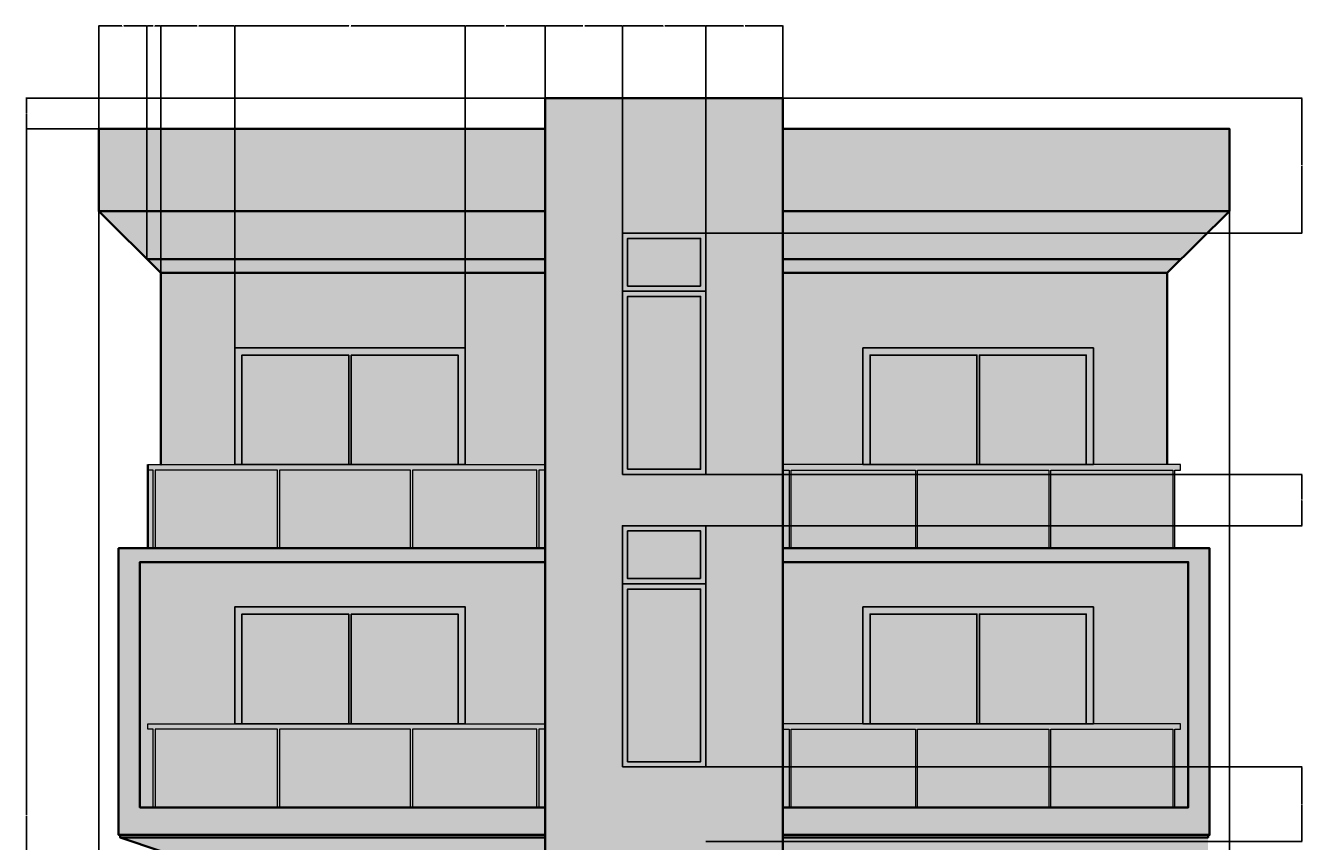
# Model space of a CAD drawing. Units: feet. Extents: x 2893 to 4112, y 897 to 1573.
# Tile 5 of 7: x 2893 to 3449, y 1217 to 1573. Entities that reach past the tile are written whole.
import ezdxf

# ---------------------------------------------------------------- set-up
doc = ezdxf.new("R2010")
doc.units = ezdxf.units.FT
for name, color, linetype, lineweight in [('A-ANNO-DIMS', 2, 'Continuous', 18), ('A-ELEV', 7, 'Continuous', 35), ('A-ELEV-PATT', 8, 'Continuous', 13), ('A-ELEV-RAIL', 4, 'Continuous', 18), ('A-GLAZ', 4, 'Continuous', 25)]:
    doc.layers.add(name, color=color, linetype=linetype, lineweight=lineweight)
doc.styles.get("Standard").update_dxf_attribs({"font": 'arial.ttf'})
doc.dimstyles.get("Standard").update_dxf_attribs({"dimtxt": 0.18, "dimasz": 0.18, "dimexe": 0.18, "dimexo": 0.0625, "dimgap": 0.09, "dimtad": 0, "dimtih": 1, "dimtoh": 1, "dimdec": 1, "dimzin": 0, "dimdsep": 46, "dimlunit": 3, "dimtxsty": 'Standard', "dimcen": 0.09, "dimadec": 0, "dimazin": 0, "dimtfac": 1, "dimtdec": 1, "dimtofl": 0, "dimtmove": 0, "dimatfit": 3, "dimfxl": 1, "dimtolj": 1, "dimtzin": 0, "dimarcsym": 0})

# ---------------------------------------------------------------- blocks, each defined once
blk = doc.blocks.new('WIN-SLIDING')
blk.add_lwpolyline([(100.48, 0), (0, 0), (0, 50.91), (100.48, 50.91)], close=True)
blk.add_lwpolyline([(100.48, 0), (0, 0), (0, 50.91), (100.48, 50.91)], close=True)
blk.add_lwpolyline([(97.33, 0), (97.33, 47.76), (50.81, 47.76), (50.81, 0), (49.67, 0), (49.67, 47.76), (3.15, 47.76), (3.15, 0)])
blk.add_lwpolyline([(97.33, 0), (97.33, 47.76), (50.81, 47.76), (50.81, 0), (49.67, 0), (49.67, 47.76), (3.15, 47.76), (3.15, 0)])
blk = doc.blocks.new('WIN-FEATURE')
for points in [[(36.35, 79.81), (0, 79.81), (0, 105.14), (36.35, 105.14)], [(36.35, 79.81), (0, 79.81), (0, 105.14), (36.35, 105.14)], [(34.08, 82.08), (2.27, 82.08), (2.27, 102.87), (34.08, 102.87)], [(34.08, 82.08), (2.27, 82.08), (2.27, 102.87), (34.08, 102.87)], [(0, 0), (36.35, 0), (36.35, 79.81), (0, 79.81)], [(0, 0), (36.35, 0), (36.35, 79.81), (0, 79.81)], [(2.27, 2.27), (34.08, 2.27), (34.08, 77.54), (2.27, 77.54)], [(2.27, 2.27), (34.08, 2.27), (34.08, 77.54), (2.27, 77.54)]]:
    blk.add_lwpolyline(points, close=True)
blk = doc.blocks.new('BALCONY-RAIL')
blk.add_lwpolyline([(56.56, 34.07), (3.3, 34.07), (3.3, 0), (2.43, 0), (2.43, 34.07), (0, 34.07), (0, 36.45), (173.25, 36.45), (173.25, 34.07), (170.48, 34.07), (170.48, 0), (169.61, 0), (169.61, 34.07), (115.47, 34.07), (115.47, 0), (114.59, 0), (114.59, 34.07), (57.43, 34.07), (57.43, 0), (56.56, 0)], close=True)
blk.add_lwpolyline([(56.56, 34.07), (3.3, 34.07), (3.3, 0), (2.43, 0), (2.43, 34.07), (0, 34.07), (0, 36.45), (173.25, 36.45), (173.25, 34.07), (170.48, 34.07), (170.48, 0), (169.61, 0), (169.61, 34.07), (115.47, 34.07), (115.47, 0), (114.59, 0), (114.59, 34.07), (57.43, 34.07), (57.43, 0), (56.56, 0)], close=True)
blk = doc.blocks.new('*D40')
at = {"layer": 'A-ANNO-DIMS', "color": 0, "lineweight": -2, "transparency": 16777216}
for p, q in [((2924.72, 1491.95), (2924.72, 1572.84)), ((2924.9, 1572.66), (2934.86, 1572.66)), ((2945.6, 1572.66), (2935.65, 1572.66)), ((2945.78, 1471.08), (2945.78, 1572.84))]:
    blk.add_line(p, q, dxfattribs=at)
at = {"layer": 'A-ANNO-DIMS', "color": 0, "transparency": 16777216}
for points in [[(2924.9, 1572.69), (2924.9, 1572.63), (2924.72, 1572.66)], [(2945.6, 1572.69), (2945.6, 1572.63), (2945.78, 1572.66)]]:
    blk.add_solid(points, dxfattribs=at)
at = {"layer": 'Defpoints', "color": 0, "transparency": 16777216}
for p in [(2945.78, 1572.66), (2924.72, 1491.89), (2945.78, 1471.01)]:
    blk.add_point(p, dxfattribs=at)
at = {"layer": 'A-ANNO-DIMS', "color": 0, "transparency": 16777216, "insert": (2935.25, 1572.66), "char_height": 0.18, "attachment_point": 5}
blk.add_mtext('\\A1;21.06', dxfattribs=at)
blk = doc.blocks.new('*D41')
at = {"layer": 'A-ANNO-DIMS', "color": 0, "lineweight": -2, "transparency": 16777216}
for p, q in [((2945.78, 1471.08), (2945.78, 1572.84)), ((2945.96, 1572.66), (2948.41, 1572.66)), ((2951.65, 1572.66), (2949.2, 1572.66)), ((2951.83, 1465.08), (2951.83, 1572.84))]:
    blk.add_line(p, q, dxfattribs=at)
at = {"layer": 'A-ANNO-DIMS', "color": 0, "transparency": 16777216}
for points in [[(2945.96, 1572.69), (2945.96, 1572.63), (2945.78, 1572.66)], [(2951.65, 1572.69), (2951.65, 1572.63), (2951.83, 1572.66)]]:
    blk.add_solid(points, dxfattribs=at)
at = {"layer": 'Defpoints', "color": 0, "transparency": 16777216}
for p in [(2951.83, 1572.66), (2945.78, 1471.01), (2951.83, 1465.01)]:
    blk.add_point(p, dxfattribs=at)
at = {"layer": 'A-ANNO-DIMS', "color": 0, "transparency": 16777216, "insert": (2948.81, 1572.66), "char_height": 0.18, "attachment_point": 5}
blk.add_mtext('\\A1;6.053', dxfattribs=at)
blk = doc.blocks.new('*D42')
at = {"layer": 'A-ANNO-DIMS', "color": 0, "lineweight": -2, "transparency": 16777216}
for p, q in [((2951.83, 1465.08), (2951.83, 1572.84)), ((2952.01, 1572.66), (2967.46, 1572.66)), ((2983.84, 1572.66), (2968.39, 1572.66)), ((2984.02, 1432.44), (2984.02, 1572.84))]:
    blk.add_line(p, q, dxfattribs=at)
at = {"layer": 'A-ANNO-DIMS', "color": 0, "transparency": 16777216}
for points in [[(2952.01, 1572.69), (2952.01, 1572.63), (2951.83, 1572.66)], [(2983.84, 1572.69), (2983.84, 1572.63), (2984.02, 1572.66)]]:
    blk.add_solid(points, dxfattribs=at)
at = {"layer": 'Defpoints', "color": 0, "transparency": 16777216}
for p in [(2984.02, 1572.66), (2951.83, 1465.01), (2984.02, 1432.38)]:
    blk.add_point(p, dxfattribs=at)
at = {"layer": 'A-ANNO-DIMS', "color": 0, "transparency": 16777216, "insert": (2967.93, 1572.66), "char_height": 0.18, "attachment_point": 5}
blk.add_mtext('\\A1;32.187', dxfattribs=at)
blk = doc.blocks.new('*D43')
at = {"layer": 'A-ANNO-DIMS', "color": 0, "lineweight": -2, "transparency": 16777216}
for p, q in [((2984.02, 1432.44), (2984.02, 1572.84)), ((2984.2, 1572.66), (3033.8, 1572.66)), ((3084.32, 1572.66), (3034.72, 1572.66)), ((3084.5, 1432.44), (3084.5, 1572.84))]:
    blk.add_line(p, q, dxfattribs=at)
at = {"layer": 'A-ANNO-DIMS', "color": 0, "transparency": 16777216}
for points in [[(2984.2, 1572.69), (2984.2, 1572.63), (2984.02, 1572.66)], [(3084.32, 1572.69), (3084.32, 1572.63), (3084.5, 1572.66)]]:
    blk.add_solid(points, dxfattribs=at)
at = {"layer": 'Defpoints', "color": 0, "transparency": 16777216}
for p in [(3084.5, 1572.66), (2984.02, 1432.38), (3084.5, 1432.38)]:
    blk.add_point(p, dxfattribs=at)
at = {"layer": 'A-ANNO-DIMS', "color": 0, "transparency": 16777216, "insert": (3034.26, 1572.66), "char_height": 0.18, "attachment_point": 5}
blk.add_mtext('\\A1;100.48', dxfattribs=at)
blk = doc.blocks.new('*D44')
at = {"layer": 'A-ANNO-DIMS', "color": 0, "lineweight": -2, "transparency": 16777216}
for p, q in [((3084.5, 1432.44), (3084.5, 1572.84)), ((3084.68, 1572.66), (3101.45, 1572.66)), ((3119.15, 1572.66), (3102.38, 1572.66)), ((3119.33, 1465.08), (3119.33, 1572.84))]:
    blk.add_line(p, q, dxfattribs=at)
at = {"layer": 'A-ANNO-DIMS', "color": 0, "transparency": 16777216}
for points in [[(3084.68, 1572.69), (3084.68, 1572.63), (3084.5, 1572.66)], [(3119.15, 1572.69), (3119.15, 1572.63), (3119.33, 1572.66)]]:
    blk.add_solid(points, dxfattribs=at)
at = {"layer": 'Defpoints', "color": 0, "transparency": 16777216}
for p in [(3119.33, 1572.66), (3119.33, 1465.01), (3084.5, 1432.38)]:
    blk.add_point(p, dxfattribs=at)
at = {"layer": 'A-ANNO-DIMS', "color": 0, "transparency": 16777216, "insert": (3101.91, 1572.66), "char_height": 0.18, "attachment_point": 5}
blk.add_mtext('\\A1;34.826', dxfattribs=at)
blk = doc.blocks.new('*D45')
at = {"layer": 'A-ANNO-DIMS', "color": 0, "lineweight": -2, "transparency": 16777216}
for p, q in [((3119.33, 1541.23), (3119.33, 1572.84)), ((3119.51, 1572.66), (3135.75, 1572.66)), ((3152.79, 1572.66), (3136.54, 1572.66)), ((3152.97, 1482.42), (3152.97, 1572.84))]:
    blk.add_line(p, q, dxfattribs=at)
at = {"layer": 'A-ANNO-DIMS', "color": 0, "transparency": 16777216}
for points in [[(3119.51, 1572.69), (3119.51, 1572.63), (3119.33, 1572.66)], [(3152.79, 1572.69), (3152.79, 1572.63), (3152.97, 1572.66)]]:
    blk.add_solid(points, dxfattribs=at)
at = {"layer": 'Defpoints', "color": 0, "transparency": 16777216}
for p in [(3152.97, 1572.66), (3119.33, 1541.16), (3152.97, 1482.36)]:
    blk.add_point(p, dxfattribs=at)
at = {"layer": 'A-ANNO-DIMS', "color": 0, "transparency": 16777216, "insert": (3136.15, 1572.66), "char_height": 0.18, "attachment_point": 5}
blk.add_mtext('\\A1;33.64', dxfattribs=at)
blk = doc.blocks.new('*D46')
at = {"layer": 'A-ANNO-DIMS', "color": 0, "lineweight": -2, "transparency": 16777216}
for p, q in [((3152.97, 1482.42), (3152.97, 1572.84)), ((3153.15, 1572.66), (3170.75, 1572.66)), ((3189.14, 1572.66), (3171.54, 1572.66)), ((3189.32, 1482.42), (3189.32, 1572.84))]:
    blk.add_line(p, q, dxfattribs=at)
at = {"layer": 'A-ANNO-DIMS', "color": 0, "transparency": 16777216}
for points in [[(3153.15, 1572.69), (3153.15, 1572.63), (3152.97, 1572.66)], [(3189.14, 1572.69), (3189.14, 1572.63), (3189.32, 1572.66)]]:
    blk.add_solid(points, dxfattribs=at)
at = {"layer": 'Defpoints', "color": 0, "transparency": 16777216}
for p in [(3189.32, 1572.66), (3152.97, 1482.36), (3189.32, 1482.36)]:
    blk.add_point(p, dxfattribs=at)
at = {"layer": 'A-ANNO-DIMS', "color": 0, "transparency": 16777216, "insert": (3171.14, 1572.66), "char_height": 0.18, "attachment_point": 5}
blk.add_mtext('\\A1;36.35', dxfattribs=at)
blk = doc.blocks.new('*D47')
at = {"layer": 'A-ANNO-DIMS', "color": 0, "lineweight": -2, "transparency": 16777216}
for p, q in [((3189.32, 1482.42), (3189.32, 1572.84)), ((3189.5, 1572.66), (3205.74, 1572.66)), ((3222.78, 1572.66), (3206.53, 1572.66)), ((3222.96, 1541.23), (3222.96, 1572.84))]:
    blk.add_line(p, q, dxfattribs=at)
at = {"layer": 'A-ANNO-DIMS', "color": 0, "transparency": 16777216}
for points in [[(3189.5, 1572.69), (3189.5, 1572.63), (3189.32, 1572.66)], [(3222.78, 1572.69), (3222.78, 1572.63), (3222.96, 1572.66)]]:
    blk.add_solid(points, dxfattribs=at)
at = {"layer": 'Defpoints', "color": 0, "transparency": 16777216}
for p in [(3222.96, 1572.66), (3222.96, 1541.16), (3189.32, 1482.36)]:
    blk.add_point(p, dxfattribs=at)
at = {"layer": 'A-ANNO-DIMS', "color": 0, "transparency": 16777216, "insert": (3206.14, 1572.66), "char_height": 0.18, "attachment_point": 5}
blk.add_mtext('\\A1;33.64', dxfattribs=at)
blk = doc.blocks.new('*D48')
at = {"layer": 'A-ANNO-DIMS', "color": 0, "lineweight": -2, "transparency": 16777216}
for p, q in [((2924.72, 1491.83), (2924.72, 897.37)), ((3417.56, 1491.83), (3417.56, 897.37)), ((2924.9, 897.55), (3170.74, 897.55)), ((3417.38, 897.55), (3171.54, 897.55))]:
    blk.add_line(p, q, dxfattribs=at)
at = {"layer": 'A-ANNO-DIMS', "color": 0, "transparency": 16777216}
for points in [[(2924.9, 897.58), (2924.9, 897.52), (2924.72, 897.55)], [(3417.38, 897.58), (3417.38, 897.52), (3417.56, 897.55)]]:
    blk.add_solid(points, dxfattribs=at)
at = {"layer": 'Defpoints', "color": 0, "transparency": 16777216}
for p in [(2924.72, 1491.89), (3417.56, 1491.89), (3417.56, 897.55)]:
    blk.add_point(p, dxfattribs=at)
at = {"layer": 'A-ANNO-DIMS', "color": 0, "transparency": 16777216, "insert": (3171.14, 897.55), "char_height": 0.18, "attachment_point": 5}
blk.add_mtext('\\A1;492.8', dxfattribs=at)
blk = doc.blocks.new('*D52')
at = {"layer": 'A-ANNO-DIMS', "color": 0, "lineweight": -2, "transparency": 16777216}
for p, q in [((3189.38, 1249.71), (3449.24, 1249.71)), ((3449.06, 1249.53), (3449.06, 1233.66)), ((3449.06, 1217.43), (3449.06, 1233.29)), ((3189.38, 1217.25), (3449.24, 1217.25))]:
    blk.add_line(p, q, dxfattribs=at)
at = {"layer": 'A-ANNO-DIMS', "color": 0, "transparency": 16777216}
for points in [[(3449.03, 1249.53), (3449.09, 1249.53), (3449.06, 1249.71)], [(3449.03, 1217.43), (3449.09, 1217.43), (3449.06, 1217.25)]]:
    blk.add_solid(points, dxfattribs=at)
at = {"layer": 'Defpoints', "color": 0, "transparency": 16777216}
for p in [(3189.32, 1249.71), (3449.06, 1249.71), (3189.32, 1217.25)]:
    blk.add_point(p, dxfattribs=at)
at = {"layer": 'A-ANNO-DIMS', "color": 0, "transparency": 16777216, "insert": (3449.06, 1233.48), "char_height": 0.18, "attachment_point": 5}
blk.add_mtext('\\A1;32.46', dxfattribs=at)
blk = doc.blocks.new('*D53')
at = {"layer": 'A-ANNO-DIMS', "color": 0, "lineweight": -2, "transparency": 16777216}
for p, q in [((3189.38, 1377.22), (3449.24, 1377.22)), ((3449.06, 1377.04), (3449.06, 1366.22)), ((3449.06, 1355.02), (3449.06, 1365.85)), ((3189.38, 1354.84), (3449.24, 1354.84))]:
    blk.add_line(p, q, dxfattribs=at)
at = {"layer": 'A-ANNO-DIMS', "color": 0, "transparency": 16777216}
for points in [[(3449.03, 1377.04), (3449.09, 1377.04), (3449.06, 1377.22)], [(3449.03, 1355.02), (3449.09, 1355.02), (3449.06, 1354.84)]]:
    blk.add_solid(points, dxfattribs=at)
at = {"layer": 'Defpoints', "color": 0, "transparency": 16777216}
for p in [(3189.32, 1377.22), (3449.06, 1377.22), (3189.32, 1354.84)]:
    blk.add_point(p, dxfattribs=at)
at = {"layer": 'A-ANNO-DIMS', "color": 0, "transparency": 16777216, "insert": (3449.06, 1366.03), "char_height": 0.18, "attachment_point": 5}
blk.add_mtext('\\A1;22.38', dxfattribs=at)
blk = doc.blocks.new('*D54')
at = {"layer": 'A-ANNO-DIMS', "color": 0, "lineweight": -2, "transparency": 16777216}
for p, q in [((3223.02, 1541.16), (3449.24, 1541.16)), ((3449.06, 1540.98), (3449.06, 1511.95)), ((3449.06, 1482.54), (3449.06, 1511.58)), ((3189.38, 1482.36), (3449.24, 1482.36))]:
    blk.add_line(p, q, dxfattribs=at)
at = {"layer": 'A-ANNO-DIMS', "color": 0, "transparency": 16777216}
for points in [[(3449.03, 1540.98), (3449.09, 1540.98), (3449.06, 1541.16)], [(3449.03, 1482.54), (3449.09, 1482.54), (3449.06, 1482.36)]]:
    blk.add_solid(points, dxfattribs=at)
at = {"layer": 'Defpoints', "color": 0, "transparency": 16777216}
for p in [(3222.96, 1541.16), (3449.06, 1541.16), (3189.32, 1482.36)]:
    blk.add_point(p, dxfattribs=at)
at = {"layer": 'A-ANNO-DIMS', "color": 0, "transparency": 16777216, "insert": (3449.06, 1511.76), "char_height": 0.18, "attachment_point": 5}
blk.add_mtext('\\A1;58.8', dxfattribs=at)
blk = doc.blocks.new('*D55')
at = {"layer": 'A-ANNO-DIMS', "color": 0, "lineweight": -2, "transparency": 16777216}
for p, q in [((2924.66, 1527.89), (2893.04, 1527.89)), ((2893.22, 1527.71), (2893.22, 1228.65)), ((2893.22, 929.23), (2893.22, 1228.29)), ((2926.44, 929.05), (2893.04, 929.05))]:
    blk.add_line(p, q, dxfattribs=at)
at = {"layer": 'A-ANNO-DIMS', "color": 0, "transparency": 16777216}
for points in [[(2893.19, 1527.71), (2893.25, 1527.71), (2893.22, 1527.89)], [(2893.19, 929.23), (2893.25, 929.23), (2893.22, 929.05)]]:
    blk.add_solid(points, dxfattribs=at)
at = {"layer": 'Defpoints', "color": 0, "transparency": 16777216}
for p in [(2893.22, 1527.89), (2924.72, 1527.89), (2926.51, 929.05)]:
    blk.add_point(p, dxfattribs=at)
at = {"layer": 'A-ANNO-DIMS', "color": 0, "transparency": 16777216, "insert": (2893.22, 1228.47), "char_height": 0.18, "attachment_point": 5}
blk.add_mtext('\\A1;598.8', dxfattribs=at)
blk = doc.blocks.new('*D56')
at = {"layer": 'A-ANNO-DIMS', "color": 0, "lineweight": -2, "transparency": 16777216}
for p, q in [((3119.26, 1541.16), (2893.04, 1541.16)), ((2893.22, 1540.98), (2893.22, 1534.71)), ((2893.22, 1528.07), (2893.22, 1534.34)), ((2924.66, 1527.89), (2893.04, 1527.89))]:
    blk.add_line(p, q, dxfattribs=at)
at = {"layer": 'A-ANNO-DIMS', "color": 0, "transparency": 16777216}
for points in [[(2893.19, 1540.98), (2893.25, 1540.98), (2893.22, 1541.16)], [(2893.19, 1528.07), (2893.25, 1528.07), (2893.22, 1527.89)]]:
    blk.add_solid(points, dxfattribs=at)
at = {"layer": 'Defpoints', "color": 0, "transparency": 16777216}
for p in [(3119.33, 1541.16), (2893.22, 1527.89), (2924.72, 1527.89)]:
    blk.add_point(p, dxfattribs=at)
at = {"layer": 'A-ANNO-DIMS', "color": 0, "transparency": 16777216, "insert": (2893.22, 1534.53), "char_height": 0.18, "attachment_point": 5}
blk.add_mtext('\\A1;13.276', dxfattribs=at)

msp = doc.modelspace()

# ---------------------------------------------------------------- hatches: boundary and pattern name
at = {"layer": 'A-ELEV-PATT'}
h = msp.add_hatch(color=256, dxfattribs=at)
h.dxf.hatch_style = 1
h.paths.add_polyline_path([(3222.9589, 1541.1646), (3119.3255, 1541.1646), (3119.3255, 967.0143), (3127.3151, 967.0143), (3127.3151, 1087.0143), (3214.9693, 1087.0143), (3214.9693, 1078.6766), (3214.9693, 967.0143), (3222.9589, 967.0143)])
h.paths.add_polyline_path([(3152.9675, 1482.3616), (3189.3169, 1482.3616), (3189.3169, 1457.0324), (3189.3169, 1377.2236), (3152.9675, 1377.2236), (3152.9675, 1457.0324)], flags=16)
h.paths.add_polyline_path([(3155.237, 1480.0922), (3187.0474, 1480.0922), (3187.0474, 1459.3019), (3155.237, 1459.3019)], flags=0)
h.paths.add_polyline_path([(3155.237, 1454.7629), (3187.0474, 1454.7629), (3187.0474, 1379.4931), (3155.237, 1379.4931)], flags=0)
h.paths.add_polyline_path([(3152.9675, 1354.8437), (3189.3169, 1354.8437), (3189.3169, 1329.5145), (3189.3169, 1249.7057), (3152.9675, 1249.7057), (3152.9675, 1329.5145)], flags=16)
h.paths.add_polyline_path([(3155.237, 1352.5742), (3187.0474, 1352.5742), (3187.0474, 1331.784), (3155.237, 1331.784)], flags=0)
h.paths.add_polyline_path([(3155.237, 1327.245), (3187.0474, 1327.245), (3187.0474, 1251.9752), (3155.237, 1251.9752)], flags=0)
h.paths.add_polyline_path([(3152.9675, 1217.2478), (3189.3169, 1217.2478), (3189.3169, 1191.9186), (3189.3169, 1112.1098), (3152.9675, 1112.1098), (3152.9675, 1191.9186)], flags=16)
h.paths.add_polyline_path([(3155.237, 1214.9783), (3187.0474, 1214.9783), (3187.0474, 1194.1881), (3155.237, 1194.1881)], flags=0)
h.paths.add_polyline_path([(3155.237, 1189.6491), (3187.0474, 1189.6491), (3187.0474, 1114.3793), (3155.237, 1114.3793)], flags=0)
h = msp.add_hatch(dxfattribs=at)
h.set_pattern_fill('AR-BRELM', color=256, scale=0.1)
h.set_pattern_definition([(0, (-663.002, 0), (0, 13.5484), [19.3675, -0.9525]), (0, (-663.002, 5.715), (0, 13.5484), [19.3675, -0.9525]), (0, (-657.922, 6.774), (0, 13.5484), [9.2075, -0.9525]), (0, (-657.922, 12.489), (0, 13.5484), [9.2075, -0.9525]), (90, (-663.002, 0), (-20.32, 1e-15), [5.715, -7.8334]), (90, (-663.954, 0), (-20.32, 1e-15), [5.715, -7.8334]), (90, (-657.922, 6.774), (-10.16, 6e-16), [5.715, -7.8334]), (90, (-658.874, 6.774), (-10.16, 6e-16), [5.715, -7.8334])])
h.paths.add_polyline_path([(3222.9589, 1541.1646), (3119.3255, 1541.1646), (3119.3255, 967.0143), (3127.3151, 967.0143), (3127.3151, 1087.0143), (3214.9693, 1087.0143), (3214.9693, 1078.6766), (3214.9693, 967.0143), (3222.9589, 967.0143)])
h.paths.add_polyline_path([(3152.9675, 1482.3616), (3189.3169, 1482.3616), (3189.3169, 1457.0324), (3189.3169, 1377.2236), (3152.9675, 1377.2236), (3152.9675, 1457.0324)], flags=16)
h.paths.add_polyline_path([(3155.237, 1480.0922), (3187.0474, 1480.0922), (3187.0474, 1459.3019), (3155.237, 1459.3019)], flags=0)
h.paths.add_polyline_path([(3155.237, 1454.7629), (3187.0474, 1454.7629), (3187.0474, 1379.4931), (3155.237, 1379.4931)], flags=0)
h.paths.add_polyline_path([(3152.9675, 1354.8437), (3189.3169, 1354.8437), (3189.3169, 1329.5145), (3189.3169, 1249.7057), (3152.9675, 1249.7057), (3152.9675, 1329.5145)], flags=16)
h.paths.add_polyline_path([(3155.237, 1352.5742), (3187.0474, 1352.5742), (3187.0474, 1331.784), (3155.237, 1331.784)], flags=0)
h.paths.add_polyline_path([(3155.237, 1327.245), (3187.0474, 1327.245), (3187.0474, 1251.9752), (3155.237, 1251.9752)], flags=0)
h.paths.add_polyline_path([(3152.9675, 1217.2478), (3189.3169, 1217.2478), (3189.3169, 1191.9186), (3189.3169, 1112.1098), (3152.9675, 1112.1098), (3152.9675, 1191.9186)], flags=16)
h.paths.add_polyline_path([(3155.237, 1214.9783), (3187.0474, 1214.9783), (3187.0474, 1194.1881), (3155.237, 1194.1881)], flags=0)
h.paths.add_polyline_path([(3155.237, 1189.6491), (3187.0474, 1189.6491), (3187.0474, 1114.3793), (3155.237, 1114.3793)], flags=0)
h = msp.add_hatch(color=256, dxfattribs=at)
h.dxf.hatch_style = 1
h.paths.add_polyline_path([(3119.3255, 1527.889), (2924.7207, 1527.889), (2924.7207, 1491.889), (3119.3255, 1491.889)])
h.paths.add_polyline_path([(3417.5637, 1527.889), (3222.9589, 1527.889), (3222.9589, 1491.889), (3417.5637, 1491.889)])
h.paths.add_polyline_path([(3119.3255, 1102.9302), (2946.0771, 1102.9302), (2946.0771, 1139.3799), (2934.0287, 1139.3799), (2934.0287, 1093.0143), (3119.3255, 1093.0143)])
h.paths.add_polyline_path([(3119.3255, 1093.0143), (2934.4679, 1093.0143), (2934.4679, 1087.0143), (3119.3255, 1087.0143)])
h.paths.add_polyline_path([(3408.2557, 1139.3799), (3396.2073, 1139.3799), (3396.2073, 1136.9984), (3396.2073, 1102.9302), (3222.9589, 1102.9302), (3222.9589, 1093.0143), (3408.2557, 1093.0143)])
h.paths.add_polyline_path([(3407.8165, 1093.0143), (3222.9589, 1093.0143), (3222.9589, 1087.0143), (3407.8165, 1087.0143)])
h = msp.add_hatch(color=256, dxfattribs=at)
h.dxf.hatch_style = 1
h.paths.add_polyline_path([(3119.3255, 1491.889), (2924.7207, 1491.889), (2945.7801, 1471.0143), (3119.3255, 1471.0143)])
h.paths.add_polyline_path([(3119.3255, 1471.0143), (2945.7801, 1471.0143), (2951.8333, 1465.0143), (3119.3255, 1465.0143)])
h.paths.add_polyline_path([(3119.3255, 1465.0143), (2951.8333, 1465.0143), (2951.8333, 1381.4641), (2984.02, 1381.4641), (2984.02, 1432.3761), (3084.4999, 1432.3761), (3084.4999, 1381.4641), (3119.3255, 1381.4641)])
h.paths.add_polyline_path([(3417.5637, 1491.889), (3222.9589, 1491.889), (3222.9589, 1471.0143), (3396.5042, 1471.0143)])
h.paths.add_polyline_path([(3396.5042, 1471.0143), (3222.9589, 1471.0143), (3222.9589, 1465.0143), (3390.4511, 1465.0143)])
h.paths.add_polyline_path([(3390.4511, 1465.0143), (3222.9589, 1465.0143), (3222.9589, 1381.4641), (3257.7845, 1381.4641), (3257.7845, 1432.3761), (3358.2644, 1432.3761), (3358.2644, 1381.4641), (3390.4511, 1381.4641)])
h.paths.add_polyline_path([(3119.3255, 1339.0143), (2942.6825, 1339.0143), (2942.6825, 1232.1197), (2948.5078, 1232.1197), (2948.5078, 1266.188), (2946.0771, 1266.188), (2946.0771, 1268.5695), (2984.02, 1268.5695), (2984.02, 1319.4815), (3084.4999, 1319.4815), (3084.4999, 1268.5695), (3119.3255, 1268.5695)], flags=17)
h.paths.add_polyline_path([(3399.6019, 1339.0143), (3222.9589, 1339.0143), (3222.9589, 1268.5695), (3257.7845, 1268.5695), (3257.7845, 1319.4815), (3358.2644, 1319.4815), (3358.2644, 1268.5695), (3396.2073, 1268.5695), (3396.2073, 1266.188), (3393.7766, 1266.188), (3393.7766, 1232.1197), (3399.6019, 1232.1197)], flags=17)
h.paths.add_polyline_path([(2942.6825, 1339.0143), (3119.3255, 1339.0143), (3119.3255, 1345.0143), (2933.3946, 1345.0143), (2933.3946, 1232.1197), (2933.3946, 1220.0947), (3119.3255, 1220.0947), (3119.3255, 1232.1197), (2942.6825, 1232.1197)])
h.paths.add_polyline_path([(3408.8898, 1345.0143), (3222.9589, 1345.0143), (3222.9589, 1339.0143), (3399.6019, 1339.0143), (3399.6019, 1232.1197), (3393.7766, 1232.1197), (3392.9028, 1232.1197), (3222.9589, 1232.1197), (3222.9589, 1220.0947), (3408.8898, 1220.0947), (3408.8898, 1232.1197)])
h.paths.add_polyline_path([(2984.02, 1190.2919), (3084.4999, 1190.2919), (3084.4999, 1139.3799), (3119.3255, 1139.3799), (3119.3255, 1213.0143), (2951.8333, 1213.0143), (2951.8333, 1139.3799), (2984.02, 1139.3799)])
h.paths.add_polyline_path([(3119.3255, 1219.0143), (2934.0287, 1219.0143), (2951.8333, 1213.0143), (3119.3255, 1213.0143)])
h.paths.add_polyline_path([(3390.4511, 1213.0143), (3222.9589, 1213.0143), (3222.9589, 1139.3799), (3257.7845, 1139.3799), (3257.7845, 1190.2919), (3358.2644, 1190.2919), (3358.2644, 1139.3799), (3390.4511, 1139.3799)])
h.paths.add_polyline_path([(3408.2557, 1219.0143), (3222.9589, 1219.0143), (3222.9589, 1213.0143), (3408.2557, 1213.0143)])
h = msp.add_hatch(color=256, dxfattribs=at)
h.dxf.hatch_style = 1
h.paths.add_polyline_path([(3119.3255, 1139.3799), (2946.0771, 1139.3799), (2946.0771, 1136.9984), (2948.5078, 1136.9984), (2948.5078, 1102.9302), (2949.3816, 1102.9302), (2949.3816, 1136.9984), (3002.6337, 1136.9984), (3002.6337, 1102.9302), (3003.5075, 1102.9302), (3003.5075, 1136.9984), (3060.6708, 1136.9984), (3060.6708, 1102.9302), (3061.5445, 1102.9302), (3061.5445, 1136.9984), (3115.685, 1136.9984), (3115.685, 1102.9302), (3116.5588, 1102.9302), (3116.5588, 1136.9984), (3119.3255, 1136.9984)])
h.paths.add_polyline_path([(2987.1701, 1187.1419), (3033.6877, 1187.1419), (3033.6877, 1139.3799), (3034.8322, 1139.3799), (3034.8322, 1187.1419), (3081.3499, 1187.1419), (3081.3499, 1139.3799), (3084.4999, 1139.3799), (3084.4999, 1190.2919), (2984.02, 1190.2919), (2984.02, 1139.3799), (2987.1701, 1139.3799)])
h.paths.add_polyline_path([(2987.1701, 1316.3314), (3033.6877, 1316.3314), (3033.6877, 1268.5695), (3034.8322, 1268.5695), (3034.8322, 1316.3314), (3081.3499, 1316.3314), (3081.3499, 1268.5695), (3084.4999, 1268.5695), (3084.4999, 1319.4815), (2984.02, 1319.4815), (2984.02, 1268.5695), (2987.1701, 1268.5695)])
h.paths.add_polyline_path([(3003.5075, 1266.188), (3060.6708, 1266.188), (3060.6708, 1232.1197), (3061.5445, 1232.1197), (3061.5445, 1266.188), (3115.685, 1266.188), (3115.685, 1232.1197), (3116.5588, 1232.1197), (3116.5588, 1266.188), (3119.3255, 1266.188), (3119.3255, 1268.5695), (2946.0771, 1268.5695), (2946.0771, 1266.188), (2948.5078, 1266.188), (2948.5078, 1232.1197), (2949.3816, 1232.1197), (2949.3816, 1266.188), (3002.6337, 1266.188), (3002.6337, 1232.1197), (3003.5075, 1232.1197)])
h.paths.add_polyline_path([(2987.1701, 1429.226), (3033.6877, 1429.226), (3033.6877, 1381.4641), (3034.8322, 1381.4641), (3034.8322, 1429.226), (3081.3499, 1429.226), (3081.3499, 1381.4641), (3084.4999, 1381.4641), (3084.4999, 1432.3761), (2984.02, 1432.3761), (2984.02, 1381.4641), (2987.1701, 1381.4641)])
h.paths.add_polyline_path([(3119.3255, 1381.4641), (2946.0771, 1381.4641), (2946.0771, 1379.0826), (2948.5078, 1379.0826), (2948.5078, 1345.0143), (2949.3816, 1345.0143), (2949.3816, 1379.0826), (3002.6337, 1379.0826), (3002.6337, 1345.0143), (3003.5075, 1345.0143), (3003.5075, 1379.0826), (3060.6708, 1379.0826), (3060.6708, 1345.0143), (3061.5445, 1345.0143), (3061.5445, 1379.0826), (3115.685, 1379.0826), (3115.685, 1345.0143), (3116.5588, 1345.0143), (3116.5588, 1379.0826), (3119.3255, 1379.0826)])
h.paths.add_polyline_path([(3189.3169, 1482.3616), (3152.9675, 1482.3616), (3152.9675, 1457.0324), (3189.3169, 1457.0324)])
h.paths.add_polyline_path([(3155.237, 1480.0922), (3187.0474, 1480.0922), (3187.0474, 1459.3019), (3155.237, 1459.3019)], flags=16)
h.paths.add_polyline_path([(3189.3169, 1457.0324), (3152.9675, 1457.0324), (3152.9675, 1377.2236), (3189.3169, 1377.2236)])
h.paths.add_polyline_path([(3155.237, 1454.7629), (3187.0474, 1454.7629), (3187.0474, 1379.4931), (3155.237, 1379.4931)], flags=16)
h.paths.add_polyline_path([(3358.2644, 1432.3761), (3257.7845, 1432.3761), (3257.7845, 1381.4641), (3260.9345, 1381.4641), (3260.9345, 1429.226), (3307.4522, 1429.226), (3307.4522, 1381.4641), (3308.5967, 1381.4641), (3308.5967, 1429.226), (3355.1143, 1429.226), (3355.1143, 1381.4641), (3358.2644, 1381.4641)])
h.paths.add_polyline_path([(3396.2073, 1381.4641), (3222.9589, 1381.4641), (3222.9589, 1379.0826), (3225.7256, 1379.0826), (3225.7256, 1345.0143), (3226.5994, 1345.0143), (3226.5994, 1379.0826), (3280.7398, 1379.0826), (3280.7398, 1345.0143), (3281.6136, 1345.0143), (3281.6136, 1379.0826), (3338.7769, 1379.0826), (3338.7769, 1345.0143), (3339.6507, 1345.0143), (3339.6507, 1379.0826), (3392.9028, 1379.0826), (3392.9028, 1345.0143), (3393.7766, 1345.0143), (3393.7766, 1379.0826), (3396.2073, 1379.0826)])
h.paths.add_polyline_path([(3358.2644, 1319.4815), (3257.7845, 1319.4815), (3257.7845, 1268.5695), (3260.9345, 1268.5695), (3260.9345, 1316.3314), (3307.4522, 1316.3314), (3307.4522, 1268.5695), (3308.5967, 1268.5695), (3308.5967, 1316.3314), (3355.1143, 1316.3314), (3355.1143, 1268.5695), (3358.2644, 1268.5695)])
h.paths.add_polyline_path([(3396.2073, 1268.5695), (3222.9589, 1268.5695), (3222.9589, 1266.188), (3225.7256, 1266.188), (3225.7256, 1232.1197), (3226.5994, 1232.1197), (3226.5994, 1266.188), (3280.7398, 1266.188), (3280.7398, 1232.1197), (3281.6136, 1232.1197), (3281.6136, 1266.188), (3338.7769, 1266.188), (3338.7769, 1232.1197), (3339.6507, 1232.1197), (3339.6507, 1266.188), (3392.9028, 1266.188), (3392.9028, 1232.1197), (3393.7766, 1232.1197), (3393.7766, 1266.188), (3396.2073, 1266.188)])
h.paths.add_polyline_path([(3260.9345, 1187.1419), (3307.4522, 1187.1419), (3307.4522, 1139.3799), (3308.5967, 1139.3799), (3308.5967, 1187.1419), (3355.1143, 1187.1419), (3355.1143, 1139.3799), (3358.2644, 1139.3799), (3358.2644, 1190.2919), (3257.7845, 1190.2919), (3257.7845, 1139.3799), (3260.9345, 1139.3799)])
h.paths.add_polyline_path([(3396.2073, 1139.3799), (3222.9589, 1139.3799), (3222.9589, 1136.9984), (3225.7256, 1136.9984), (3225.7256, 1102.9302), (3226.5994, 1102.9302), (3226.5994, 1136.9984), (3280.7398, 1136.9984), (3280.7398, 1102.9302), (3281.6136, 1102.9302), (3281.6136, 1136.9984), (3338.7769, 1136.9984), (3338.7769, 1102.9302), (3339.6507, 1102.9302), (3339.6507, 1136.9984), (3392.9028, 1136.9984), (3392.9028, 1102.9302), (3393.7766, 1102.9302), (3393.7766, 1136.9984), (3396.2073, 1136.9984)])
h.paths.add_polyline_path([(3189.3169, 1354.8437), (3152.9675, 1354.8437), (3152.9675, 1329.5145), (3189.3169, 1329.5145)])
h.paths.add_polyline_path([(3155.237, 1331.784), (3155.237, 1352.5742), (3187.0474, 1352.5742), (3187.0474, 1331.784)], flags=16)
h.paths.add_polyline_path([(3189.3169, 1329.5145), (3152.9675, 1329.5145), (3152.9675, 1249.7057), (3189.3169, 1249.7057)])
h.paths.add_polyline_path([(3155.237, 1327.245), (3187.0474, 1327.245), (3187.0474, 1251.9752), (3155.237, 1251.9752)], flags=16)
h.paths.add_polyline_path([(3189.3169, 1191.9186), (3152.9675, 1191.9186), (3152.9675, 1112.1098), (3189.3169, 1112.1098)])
h.paths.add_polyline_path([(3155.237, 1189.6491), (3187.0474, 1189.6491), (3187.0474, 1114.3793), (3155.237, 1114.3793)], flags=16)
h.paths.add_polyline_path([(3189.3169, 1217.2478), (3152.9675, 1217.2478), (3152.9675, 1191.9186), (3189.3169, 1191.9186)])
h.paths.add_polyline_path([(3155.237, 1194.1881), (3155.237, 1214.9783), (3187.0474, 1214.9783), (3187.0474, 1194.1881)], flags=16)
h = msp.add_hatch(color=256, dxfattribs=at)
h.dxf.hatch_style = 1
h.paths.add_polyline_path([(3033.6877, 1429.226), (2987.1701, 1429.226), (2987.1701, 1381.4641), (3033.6877, 1381.4641)])
h.paths.add_polyline_path([(3081.3499, 1429.226), (3034.8322, 1429.226), (3034.8322, 1381.4641), (3081.3499, 1381.4641)])
h.paths.add_polyline_path([(3115.685, 1379.0826), (3061.5445, 1379.0826), (3061.5445, 1345.0143), (3115.685, 1345.0143)])
h.paths.add_polyline_path([(3119.3255, 1379.0826), (3116.5588, 1379.0826), (3116.5588, 1345.0143), (3119.3255, 1345.0143)])
h.paths.add_polyline_path([(3060.6708, 1379.0826), (3003.5075, 1379.0826), (3003.5075, 1345.0143), (3060.6708, 1345.0143)])
h.paths.add_polyline_path([(3002.6337, 1379.0826), (2949.3816, 1379.0826), (2949.3816, 1345.0143), (3002.6337, 1345.0143)])
h.paths.add_polyline_path([(2948.5078, 1379.0826), (2946.0771, 1379.0826), (2946.0771, 1345.0143), (2948.5078, 1345.0143)])
h.paths.add_polyline_path([(3355.1143, 1429.226), (3308.5967, 1429.226), (3308.5967, 1381.4641), (3355.1143, 1381.4641)])
h.paths.add_polyline_path([(3307.4522, 1429.226), (3260.9345, 1429.226), (3260.9345, 1381.4641), (3307.4522, 1381.4641)])
h.paths.add_polyline_path([(3225.7256, 1379.0826), (3222.9589, 1379.0826), (3222.9589, 1345.0143), (3225.7256, 1345.0143)])
h.paths.add_polyline_path([(3280.7398, 1379.0826), (3226.5994, 1379.0826), (3226.5994, 1345.0143), (3280.7398, 1345.0143)])
h.paths.add_polyline_path([(3338.7769, 1379.0826), (3281.6136, 1379.0826), (3281.6136, 1345.0143), (3338.7769, 1345.0143)])
h.paths.add_polyline_path([(3392.9028, 1379.0826), (3339.6507, 1379.0826), (3339.6507, 1345.0143), (3392.9028, 1345.0143)])
h.paths.add_polyline_path([(3187.0474, 1480.0922), (3155.237, 1480.0922), (3155.237, 1459.3019), (3187.0474, 1459.3019)])
h.paths.add_polyline_path([(3187.0474, 1454.7629), (3155.237, 1454.7629), (3155.237, 1379.4931), (3187.0474, 1379.4931)])
h.paths.add_polyline_path([(3187.0474, 1352.5742), (3155.237, 1352.5742), (3155.237, 1331.784), (3187.0474, 1331.784)])
h.paths.add_polyline_path([(3187.0474, 1327.245), (3155.237, 1327.245), (3155.237, 1251.9752), (3187.0474, 1251.9752)])
h.paths.add_polyline_path([(3033.6877, 1316.3314), (2987.1701, 1316.3314), (2987.1701, 1268.5695), (3033.6877, 1268.5695)])
h.paths.add_polyline_path([(3081.3499, 1316.3314), (3034.8322, 1316.3314), (3034.8322, 1268.5695), (3081.3499, 1268.5695)])
h.paths.add_polyline_path([(3002.6337, 1266.188), (2949.3816, 1266.188), (2949.3816, 1232.1197), (3002.6337, 1232.1197)])
h.paths.add_polyline_path([(3060.6708, 1266.188), (3003.5075, 1266.188), (3003.5075, 1232.1197), (3060.6708, 1232.1197)])
h.paths.add_polyline_path([(3115.685, 1266.188), (3061.5445, 1266.188), (3061.5445, 1232.1197), (3115.685, 1232.1197)])
h.paths.add_polyline_path([(3119.3255, 1266.188), (3116.5588, 1266.188), (3116.5588, 1232.1197), (3119.3255, 1232.1197)])
h.paths.add_polyline_path([(3307.4522, 1316.3314), (3260.9345, 1316.3314), (3260.9345, 1268.5695), (3307.4522, 1268.5695)])
h.paths.add_polyline_path([(3355.1143, 1316.3314), (3308.5967, 1316.3314), (3308.5967, 1268.5695), (3355.1143, 1268.5695)])
h.paths.add_polyline_path([(3392.9028, 1266.188), (3339.6507, 1266.188), (3339.6507, 1232.1197), (3392.9028, 1232.1197)])
h.paths.add_polyline_path([(3338.7769, 1266.188), (3281.6136, 1266.188), (3281.6136, 1232.1197), (3338.7769, 1232.1197)])
h.paths.add_polyline_path([(3280.7398, 1266.188), (3226.5994, 1266.188), (3226.5994, 1232.1197), (3280.7398, 1232.1197)])
h.paths.add_polyline_path([(3225.7256, 1266.188), (3222.9589, 1266.188), (3222.9589, 1232.1197), (3225.7256, 1232.1197)])
h.paths.add_polyline_path([(3033.6877, 1187.1419), (2987.1701, 1187.1419), (2987.1701, 1139.3799), (3033.6877, 1139.3799)])
h.paths.add_polyline_path([(3081.3499, 1187.1419), (3034.8322, 1187.1419), (3034.8322, 1139.3799), (3081.3499, 1139.3799)])
h.paths.add_polyline_path([(3002.6337, 1136.9984), (2949.3816, 1136.9984), (2949.3816, 1102.9302), (3002.6337, 1102.9302)])
h.paths.add_polyline_path([(3060.6708, 1136.9984), (3003.5075, 1136.9984), (3003.5075, 1102.9302), (3060.6708, 1102.9302)])
h.paths.add_polyline_path([(3115.685, 1136.9984), (3061.5445, 1136.9984), (3061.5445, 1102.9302), (3115.685, 1102.9302)])
h.paths.add_polyline_path([(3187.0474, 1214.9783), (3155.237, 1214.9783), (3155.237, 1194.1881), (3187.0474, 1194.1881)])
h.paths.add_polyline_path([(3187.0474, 1189.6491), (3155.237, 1189.6491), (3155.237, 1114.3793), (3187.0474, 1114.3793)])
h.paths.add_polyline_path([(3307.4522, 1187.1419), (3260.9345, 1187.1419), (3260.9345, 1139.3799), (3307.4522, 1139.3799)])
h.paths.add_polyline_path([(3355.1143, 1187.1419), (3308.5967, 1187.1419), (3308.5967, 1139.3799), (3355.1143, 1139.3799)])
h.paths.add_polyline_path([(3280.7398, 1136.9984), (3226.5994, 1136.9984), (3226.5994, 1102.9302), (3280.7398, 1102.9302)])
h.paths.add_polyline_path([(3338.7769, 1136.9984), (3281.6136, 1136.9984), (3281.6136, 1102.9302), (3338.7769, 1102.9302)])
h.paths.add_polyline_path([(3392.9028, 1136.9984), (3339.6507, 1136.9984), (3339.6507, 1102.9302), (3392.9028, 1102.9302)])
h.paths.add_polyline_path([(3225.7256, 1136.9984), (3222.9589, 1136.9984), (3222.9589, 1102.9302), (3225.7256, 1102.9302)])
h.paths.add_polyline_path([(3119.3255, 1136.9984), (3116.5588, 1136.9984), (3116.5588, 1102.9302), (3119.3255, 1102.9302)])
h.paths.add_polyline_path([(2948.5078, 1136.9984), (2946.0771, 1136.9984), (2946.0771, 1102.9302), (2948.5078, 1102.9302)])
h.paths.add_polyline_path([(3396.2073, 1136.9984), (3393.7766, 1136.9984), (3393.7766, 1102.9302), (3396.2073, 1102.9302)])

# ---------------------------------------------------------------- linework, layer by layer
at = {"layer": 'A-ELEV'}
for p, q in [((3119.3255, 967.0143), (3119.3255, 1541.1646)), ((3119.3255, 1541.1646), (3222.9589, 1541.1646)), ((3222.9589, 967.0143), (3222.9589, 1541.1646)), ((2924.7207, 1491.889), (2924.7207, 1527.889)), ((2924.7207, 1527.889), (3119.3255, 1527.889)), ((3222.9589, 1527.889), (3417.5637, 1527.889)), ((3417.5637, 1491.889), (3417.5637, 1527.889)), ((2951.8333, 1465.0143), (2924.7207, 1491.889)), ((2924.7207, 1491.889), (3119.3255, 1491.889)), ((3417.5637, 1491.889), (3222.9589, 1491.889)), ((3417.5637, 1491.889), (3222.9589, 1491.889)), ((3390.4511, 1465.0143), (3417.5637, 1491.889)), ((3119.3255, 1471.0143), (2945.7801, 1471.0143)), ((3119.3255, 1471.0143), (2945.7801, 1471.0143)), ((3396.5042, 1471.0143), (3222.9589, 1471.0143)), ((3396.5042, 1471.0143), (3222.9589, 1471.0143)), ((2951.8333, 1465.0143), (3119.3255, 1465.0143)), ((2951.8333, 1381.4641), (2951.8333, 1465.0143)), ((2951.8333, 1465.0143), (2951.8333, 1381.4641)), ((3222.9589, 1465.0143), (3390.4511, 1465.0143)), ((3222.9589, 1465.0143), (3390.4511, 1465.0143)), ((3390.4511, 1465.0143), (3390.4511, 1381.4641)), ((2946.0771, 1381.4641), (2946.0771, 1345.0143)), ((2946.0771, 1381.4641), (2946.0771, 1345.0143)), ((2933.3946, 1220.0947), (2933.3946, 1345.0143)), ((3119.3255, 1345.0143), (2933.3946, 1345.0143)), ((3119.3255, 1345.0143), (2933.3946, 1345.0143)), ((3408.8898, 1345.0143), (3222.9589, 1345.0143)), ((3408.8898, 1345.0143), (3222.9589, 1345.0143)), ((3408.8898, 1220.0947), (3408.8898, 1345.0143)), ((2942.6825, 1339.0143), (3119.3255, 1339.0143)), ((3222.9589, 1339.0143), (3399.6019, 1339.0143)), ((2934.0287, 1220.0947), (2933.3946, 1220.0947)), ((2934.0287, 1219.0143), (2934.0287, 1220.0947)), ((2951.8333, 1213.0143), (2934.0287, 1219.0143)), ((3119.3255, 1219.0143), (2934.0287, 1219.0143)), ((3119.3255, 1219.0143), (2934.0287, 1219.0143)), ((3408.2557, 1219.0143), (3222.9589, 1219.0143)), ((3408.2557, 1219.0143), (3222.9589, 1219.0143))]:
    msp.add_line(p, q, dxfattribs=at)
for points in [[(3119.3255, 967.0143), (3119.3255, 1541.1646), (3222.9589, 1541.1646), (3222.9589, 967.0143)], [(3119.3255, 1491.889), (2924.7207, 1491.889), (2924.7207, 1527.889), (3119.3255, 1527.889)], [(3222.9589, 1527.889), (3417.5637, 1527.889), (3417.5637, 1491.889), (3390.4511, 1465.0143), (3390.4511, 1381.4641)], [(3119.3255, 1465.0143), (2951.8333, 1465.0143), (2951.8333, 1381.4641), (2951.8333, 1465.0143), (2924.7207, 1491.889)], [(2933.3946, 1232.1197), (2933.3946, 1345.0143)], [(3119.3255, 1339.0143), (2942.6825, 1339.0143), (2942.6825, 1232.1197), (3119.3255, 1232.1197), (3119.3255, 1220.0947), (2933.3946, 1220.0947), (2933.3946, 1232.1197), (2933.3946, 1345.0143), (2933.3946, 1220.0947), (2934.0287, 1220.0947), (2934.0287, 1219.0143), (2951.8333, 1213.0143), (2951.8333, 1139.3799), (2951.8333, 1213.0143), (3119.3255, 1213.0143)], [(3399.6019, 1220.0947), (3408.8898, 1220.0947), (3408.8898, 1345.0143)], [(3399.6019, 1220.0947), (3408.8898, 1220.0947), (3408.8898, 1345.0143), (3408.8898, 1220.0947)], [(2942.6825, 1339.0143), (2942.6825, 1232.1197)], [(3408.8898, 1232.1197), (3408.8898, 1220.0947), (3222.9589, 1220.0947), (3222.9589, 1232.1197), (3399.6019, 1232.1197), (3399.6019, 1339.0143), (3222.9589, 1339.0143)], [(3399.6019, 1339.0143), (3399.6019, 1232.1197)], [(2933.3946, 1232.1197), (2933.3946, 1220.0947), (3119.3255, 1220.0947), (3119.3255, 1232.1197), (2942.6825, 1232.1197)], [(3408.8898, 1232.1197), (3408.8898, 1220.0947), (3222.9589, 1220.0947), (3222.9589, 1232.1197), (3399.6019, 1232.1197)]]:
    msp.add_lwpolyline(points, dxfattribs=at)
for points in [[(3119.3255, 1219.0143), (2934.0287, 1219.0143), (2934.0287, 1220.0947), (3119.3255, 1220.0947)], [(3119.3255, 1219.0143), (2934.0287, 1219.0143), (2934.0287, 1220.0947), (3119.3255, 1220.0947)], [(3222.9589, 1219.0143), (3408.2557, 1219.0143), (3408.2557, 1220.0947), (3222.9589, 1220.0947)], [(3222.9589, 1219.0143), (3408.2557, 1219.0143), (3408.2557, 1220.0947), (3222.9589, 1220.0947)]]:
    msp.add_lwpolyline(points, close=True, dxfattribs=at)

# ---------------------------------------------------------------- block references
at = {"layer": 'A-ELEV-RAIL'}
for p in [(2946.077, 1345.0142), (2946.077, 1232.1195)]:
    msp.add_blockref('BALCONY-RAIL', p, dxfattribs=at)
at = {"layer": 'A-ELEV-RAIL', "extrusion": (0, 0, -1), "zscale": -1}
for p in [(-3396.2074, 1345.0142), (-3396.2074, 1232.1195)]:
    msp.add_blockref('BALCONY-RAIL', p, dxfattribs=at)
at = {"layer": 'A-GLAZ'}
for name, p in [('WIN-FEATURE', (3152.967, 1377.2238)), ('WIN-SLIDING', (2984.02, 1381.4642)), ('WIN-FEATURE', (3152.967, 1249.7059)), ('WIN-SLIDING', (2984.02, 1268.5695))]:
    msp.add_blockref(name, p, dxfattribs=at)
at = {"layer": 'A-GLAZ', "extrusion": (0, 0, -1), "zscale": -1}
for p in [(-3358.2644, 1381.4642), (-3358.2644, 1268.5695)]:
    msp.add_blockref('WIN-SLIDING', p, dxfattribs=at)

# ---------------------------------------------------------------- dimensions: what is measured, and where the dimension line sits
at = {"layer": 'A-ANNO-DIMS'}
for base, p1, p2, override, picture, middle in [((2945.7801, 1572.6646), (2924.7207, 1491.889), (2945.7801, 1471.0143), {"dimdec": 2, "dimlfac": 1, "dimrnd": 0, "dimzin": 0, "dimdsep": 46, "dimlunit": 2}, '*D40', (2935.2504, 1572.6646)), ((2951.8333, 1572.6646), (2945.7801, 1471.0143), (2951.8333, 1465.0143), {"dimdec": 3, "dimlfac": 1, "dimrnd": 0, "dimzin": 0, "dimdsep": 46, "dimlunit": 2}, '*D41', (2948.8067, 1572.6646)), ((2984.02, 1572.6646), (2951.8333, 1465.0143), (2984.02, 1432.3761), {"dimdec": 3, "dimlfac": 1, "dimrnd": 0, "dimzin": 0, "dimdsep": 46, "dimlunit": 2}, '*D42', (2967.9266, 1572.6646)), ((3084.4999, 1572.6646), (2984.02, 1432.3761), (3084.4999, 1432.3761), {"dimdec": 2, "dimlfac": 1, "dimrnd": 0, "dimzin": 0, "dimdsep": 46, "dimlunit": 2}, '*D43', (3034.26, 1572.6646)), ((3119.3255, 1572.6646), (3084.4999, 1432.3761), (3119.3255, 1465.0143), {"dimdec": 3, "dimlfac": 1, "dimrnd": 0, "dimzin": 0, "dimdsep": 46, "dimlunit": 2}, '*D44', (3101.9127, 1572.6646)), ((3152.9675, 1572.6646), (3119.3255, 1541.1646), (3152.9675, 1482.3616), {"dimdec": 2, "dimlfac": 1, "dimrnd": 0, "dimzin": 0, "dimdsep": 46, "dimlunit": 2}, '*D45', (3136.1465, 1572.6646)), ((3189.3169, 1572.6646), (3152.9675, 1482.3616), (3189.3169, 1482.3616), {"dimdec": 2, "dimlfac": 1, "dimrnd": 0, "dimzin": 0, "dimdsep": 46, "dimlunit": 2}, '*D46', (3171.1422, 1572.6646)), ((3222.9589, 1572.6646), (3189.3169, 1482.3616), (3222.9589, 1541.1646), {"dimdec": 2, "dimlfac": 1, "dimrnd": 0, "dimzin": 0, "dimdsep": 46, "dimlunit": 2}, '*D47', (3206.1379, 1572.6646)), ((3417.5637, 897.5499), (2924.7207, 1491.889), (3417.5637, 1491.889), {"dimdec": 1, "dimlfac": 1, "dimrnd": 0, "dimzin": 0, "dimdsep": 46, "dimlunit": 2}, '*D48', (3171.1422, 897.5499))]:
    dim = msp.add_linear_dim(base=base, p1=p1, p2=p2, dimstyle='Standard', override=override, dxfattribs=at)
    dim.commit()
    dim.dimension.update_dxf_attribs({"geometry": picture, "text_midpoint": middle})
for base, p1, p2, override, picture, middle in [((2893.2207, 1527.889), (3119.3255, 1541.1646), (2924.7207, 1527.889), {"dimdec": 3, "dimlfac": 1, "dimrnd": 0, "dimzin": 0, "dimdsep": 46, "dimlunit": 2}, '*D56', (2893.2207, 1534.5268)), ((3449.0637, 1541.1646), (3189.3169, 1482.3616), (3222.9589, 1541.1646), {"dimdec": 1, "dimlfac": 1, "dimrnd": 0, "dimzin": 0, "dimdsep": 46, "dimlunit": 2}, '*D54', (3449.0637, 1511.7631)), ((2893.2207, 1527.889), (2926.5072, 929.0499), (2924.7207, 1527.889), {"dimdec": 1, "dimlfac": 1, "dimrnd": 0, "dimzin": 0, "dimdsep": 46, "dimlunit": 2}, '*D55', (2893.2207, 1228.4695)), ((3449.0637, 1377.2236), (3189.3169, 1354.8437), (3189.3169, 1377.2236), {"dimdec": 2, "dimlfac": 1, "dimrnd": 0, "dimzin": 0, "dimdsep": 46, "dimlunit": 2}, '*D53', (3449.0637, 1366.0337)), ((3449.0637, 1249.7057), (3189.3169, 1217.2478), (3189.3169, 1249.7057), {"dimdec": 2, "dimlfac": 1, "dimrnd": 0, "dimzin": 0, "dimdsep": 46, "dimlunit": 2}, '*D52', (3449.0637, 1233.4768))]:
    dim = msp.add_linear_dim(base=base, p1=p1, p2=p2, angle=90, dimstyle='Standard', override=override, dxfattribs=at)
    dim.commit()
    dim.dimension.update_dxf_attribs({"geometry": picture, "text_midpoint": middle})

doc.saveas('drawing.dxf')
